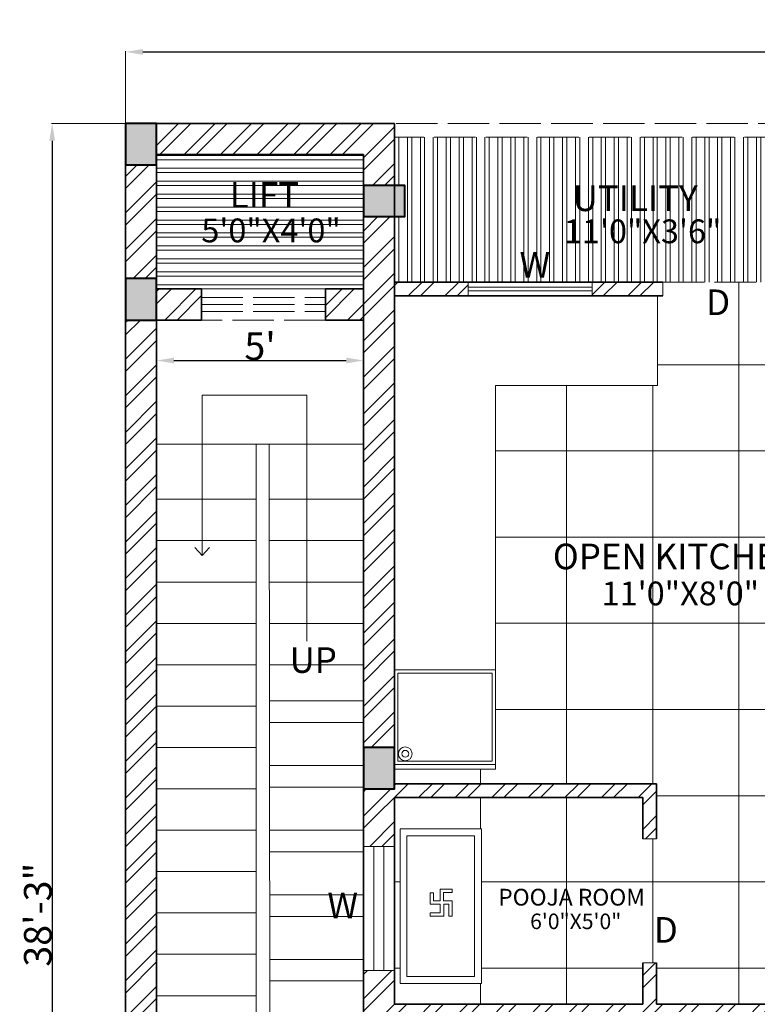
# Model space of a CAD drawing. Units: inches. Extents: x 351 to 1738, y -265 to 286.
# Tile 2 of 38: x 351 to 565, y 0 to 286. Entities that reach past the tile are written whole.
import ezdxf

# ---------------------------------------------------------------- set-up
doc = ezdxf.new("R2010")
doc.units = ezdxf.units.IN
doc.header["$MEASUREMENT"] = 0
doc.linetypes.add('ACAD_ISO02W100', pattern=[15, 12, -3])
for name, color, linetype, lineweight in [('A-ANNO-DIMS', 2, 'Continuous', 18), ('A-ANNO-SYMB', 7, 'Continuous', 18), ('A-AREA-IDEN', 7, 'Continuous', 18), ('A-COLS', 7, 'Continuous', 40), ('A-COLS-PATT', 6, 'Continuous', 13), ('A-DOOR', 3, 'Continuous', 18), ('A-DOOR-OVHD', 3, 'ACAD_ISO02W100', 13), ('A-FLOR-CASE', 9, 'Continuous', 18), ('A-FLOR-EVTR', 242, 'ACAD_ISO02W100', 18), ('A-FLOR-EVTR-PATT', 9, 'Continuous', 9), ('A-FLOR-FIXT', 9, 'Continuous', 18), ('A-FLOR-OVHD', 1, 'ACAD_ISO02W100', 18), ('A-FLOR-PATT', 9, 'Continuous', 9), ('A-FLOR-STRS', 7, 'Continuous', 18), ('A-GLAZ', 4, 'Continuous', 18), ('A-WALL', 7, 'Continuous', 35), ('A-WALL-PATT', 152, 'Continuous', 13)]:
    doc.layers.add(name, color=color, linetype=linetype, lineweight=lineweight)
doc.styles.add('Annotative', font='arial.ttf')
doc.styles.get("Standard").update_dxf_attribs({"font": 'arial.ttf'})
doc.dimstyles.get("Standard").update_dxf_attribs({"dimtxt": 8, "dimasz": 5, "dimexe": 0.18, "dimexo": 0.0625, "dimgap": 0.09, "dimtad": 1, "dimtoh": 1, "dimzin": 0, "dimdsep": 46, "dimlunit": 4, "dimtxsty": 'Standard', "dimcen": 0, "dimclre": 256, "dimadec": 0, "dimazin": 0, "dimtfac": 1, "dimtofl": 0, "dimtmove": 0, "dimatfit": 3, "dimfxl": 1, "dimtolj": 1, "dimtzin": 0, "dimlwe": -1, "dimarcsym": 0})

# ---------------------------------------------------------------- blocks, each defined once
blk = doc.blocks.new('*D2')
at = {"layer": 'A-ANNO-DIMS', "color": 0, "transparency": 16777216}
for p, q in [((382.16, 256.03), (382.16, 276.92)), ((914.16, 256.03), (914.16, 276.92))]:
    blk.add_line(p, q, dxfattribs=at)
at = {"layer": 'A-ANNO-DIMS', "color": 0, "lineweight": -2, "transparency": 16777216}
blk.add_line((387.16, 276.74), (909.16, 276.74), dxfattribs=at)
at = {"layer": 'A-ANNO-DIMS', "color": 0, "transparency": 16777216}
for points in [[(387.16, 277.57), (387.16, 275.91), (382.16, 276.74)], [(909.16, 277.57), (909.16, 275.91), (914.16, 276.74)]]:
    blk.add_solid(points, dxfattribs=at)
at = {"layer": 'Defpoints', "color": 0, "transparency": 16777216}
for p in [(914.16, 276.74), (382.16, 255.96), (914.16, 255.96)]:
    blk.add_point(p, dxfattribs=at)
at = {"layer": 'A-ANNO-DIMS', "color": 0, "transparency": 16777216, "insert": (648.16, 280.83), "char_height": 8, "attachment_point": 5}
blk.add_mtext('\\A1;44\'-4"', dxfattribs=at)
blk = doc.blocks.new('*D3')
at = {"layer": 'A-ANNO-DIMS', "color": 0, "transparency": 16777216}
for p, q in [((382.09, 255.96), (360.67, 255.96)), ((382.09, -203.04), (360.67, -203.04))]:
    blk.add_line(p, q, dxfattribs=at)
at = {"layer": 'A-ANNO-DIMS', "color": 0, "lineweight": -2, "transparency": 16777216}
blk.add_line((360.85, 250.96), (360.85, -198.04), dxfattribs=at)
at = {"layer": 'A-ANNO-DIMS', "color": 0, "transparency": 16777216}
for points in [[(360.02, 250.96), (361.69, 250.96), (360.85, 255.96)], [(360.02, -198.04), (361.69, -198.04), (360.85, -203.04)]]:
    blk.add_solid(points, dxfattribs=at)
at = {"layer": 'Defpoints', "color": 0, "transparency": 16777216}
for p in [(382.16, 255.96), (360.85, -203.04), (382.16, -203.04)]:
    blk.add_point(p, dxfattribs=at)
at = {"layer": 'A-ANNO-DIMS', "color": 0, "transparency": 16777216, "insert": (356.68, 26.46), "char_height": 8, "attachment_point": 5, "rotation": 90}
blk.add_mtext('\\A1;38\'-3"', dxfattribs=at)
blk = doc.blocks.new('*D6')
at = {"layer": 'A-ANNO-DIMS', "color": 0, "transparency": 16777216}
for p, q in [((391.16, 198.9), (391.16, 187.03)), ((451.16, 198.9), (451.16, 187.03))]:
    blk.add_line(p, q, dxfattribs=at)
at = {"layer": 'A-ANNO-DIMS', "color": 0, "lineweight": -2, "transparency": 16777216}
blk.add_line((396.16, 187.21), (446.16, 187.21), dxfattribs=at)
at = {"layer": 'A-ANNO-DIMS', "color": 0, "transparency": 16777216}
for points in [[(396.16, 188.04), (396.16, 186.37), (391.16, 187.21)], [(446.16, 188.04), (446.16, 186.37), (451.16, 187.21)]]:
    blk.add_solid(points, dxfattribs=at)
at = {"layer": 'Defpoints', "color": 0, "transparency": 16777216}
for p in [(391.16, 198.96), (451.16, 198.96), (451.16, 187.21)]:
    blk.add_point(p, dxfattribs=at)
at = {"layer": 'A-ANNO-DIMS', "color": 0, "transparency": 16777216, "insert": (421.16, 191.36), "char_height": 8, "attachment_point": 5}
blk.add_mtext("\\A1;5'", dxfattribs=at)
blk = doc.blocks.new('COL-9x12')
blk.add_lwpolyline([(0, 12), (0, 0), (9, 0), (9, 12)], close=True)
blk = doc.blocks.new('WIN-36-STAIR')
for p, q in [((3.02, 0), (3.02, 36)), ((5.92, 0), (5.92, 36))]:
    blk.add_line(p, q)
blk.add_lwpolyline([(0, 0), (0, 36), (9, 36), (9, 0)], close=True)
blk = doc.blocks.new('LIFT-DOOR-36')
for p, q in [((0, 9), (36, 9)), ((0, 6.5), (36, 6.5)), ((0, 4.5), (36, 4.5)), ((0, 2.5), (36, 2.5)), ((36, 0), (0, 0))]:
    blk.add_line(p, q)

msp = doc.modelspace()

# ---------------------------------------------------------------- hatches: boundary and pattern name
at = {"layer": 'A-COLS-PATT'}
h = msp.add_hatch(color=256, dxfattribs=at)
h.dxf.hatch_style = 1
h.paths.add_polyline_path([(460.155, 237.963), (451.155, 237.963), (451.155, 228.963), (460.155, 228.963)])
h.paths.add_polyline_path([(463.155, 237.963), (460.155, 237.963), (460.155, 228.963), (463.155, 228.963)])
h.paths.add_polyline_path([(391.155, 255.963), (382.155, 255.963), (382.155, 243.963), (391.155, 243.963)])
h.paths.add_polyline_path([(391.155, 210.963), (382.155, 210.963), (382.155, 198.963), (391.155, 198.963)])
h.paths.add_polyline_path([(391.155, -45.037), (382.155, -45.037), (382.155, -57.037), (391.155, -57.037)])
h.paths.add_polyline_path([(460.155, -45.037), (451.155, -45.037), (451.155, -57.037), (460.155, -57.037)])
h.paths.add_polyline_path([(460.155, -161.037), (451.155, -161.037), (451.155, -164.037), (451.155, -173.037), (460.155, -173.037)])
h.paths.add_polyline_path([(391.155, -161.037), (382.155, -161.037), (382.155, -173.037), (391.155, -173.037)])
h.paths.add_polyline_path([(596, -164.037), (584, -164.037), (584, -173.037), (596, -173.037)])
h.paths.add_polyline_path([(596, -50), (584, -50), (584, -59), (596, -59)])
h.paths.add_polyline_path([(596.155, 73.463), (592.155, 73.463), (592.155, 64.463), (596.155, 64.463)])
h.paths.add_polyline_path([(592.155, 73.463), (584.155, 73.463), (584.155, 64.463), (592.155, 64.463)])
h.paths.add_polyline_path([(596.155, 237.963), (584.155, 237.963), (584.155, 228.963), (596.155, 228.963)])
h.paths.add_polyline_path([(739.655, 237.963), (727.655, 237.963), (727.655, 228.963), (739.655, 228.963)])
h.paths.add_polyline_path([(883.515, 237.963), (871.515, 237.963), (871.515, 228.963), (883.515, 228.963)])
h.paths.add_polyline_path([(883.515, 73.463), (871.515, 73.463), (871.515, 64.463), (883.515, 64.463)])
h.paths.add_polyline_path([(731.655, 73.463), (727.655, 73.463), (727.655, 64.463), (731.655, 64.463)])
h.paths.add_polyline_path([(739.515, 73.463), (731.655, 73.463), (731.655, 64.463), (739.515, 64.463)])
h.paths.add_polyline_path([(883.515, -53.037), (871.515, -53.037), (871.515, -57.037), (883.515, -57.037)])
h.paths.add_polyline_path([(883.515, -48.037), (871.515, -48.037), (871.515, -53.037), (883.515, -53.037)])
h.paths.add_polyline_path([(739.515, -48.037), (727.515, -48.037), (727.515, -56.5), (727.516, -57.037), (739.515, -57.037)])
h.paths.add_polyline_path([(883.515, -164.037), (871.515, -164.037), (871.515, -173.037), (883.515, -173.037)])
h = msp.add_hatch(color=256, dxfattribs=at)
h.dxf.hatch_style = 1
h.paths.add_polyline_path([(460.155, 74.963), (451.155, 74.963), (451.155, 62.963), (460.155, 62.963)])
at = {"layer": 'A-FLOR-EVTR-PATT', "transparency": 33554559}
h = msp.add_hatch(dxfattribs=at)
h.set_pattern_fill('ANSI32', color=256, scale=10, angle=135)
h.set_pattern_definition([(180, (391.1553, 207.9627), (-2e-16, -3.75), []), (180, (389.9053, 209.2127), (-2e-16, -3.75), [])])
h.paths.add_polyline_path([(451.155, 246.963), (391.155, 246.963), (391.155, 243.963), (391.155, 207.963), (404.155, 207.963), (440.155, 207.963), (451.155, 207.963)])
at = {"layer": 'A-FLOR-PATT', "transparency": 33554559}
h = msp.add_hatch(dxfattribs=at)
h.set_pattern_fill('ANSI32', color=256, scale=10, angle=45)
h.set_pattern_definition([(90, (460.1553, 209.9627), (-3.75, 0), []), (90, (461.4053, 211.2127), (-3.75, 0), [])])
h.paths.add_polyline_path([(584.155, 237.963), (588.655, 237.963), (588.655, 251.963), (460.155, 251.963), (460.155, 237.963), (463.155, 237.963), (463.155, 228.963), (460.155, 228.963), (460.155, 209.963), (538, 209.963), (574, 209.963), (592.155, 209.963), (592.155, 228.963), (584.155, 228.963)])
h = msp.add_hatch(dxfattribs=at)
h.set_pattern_fill('ANSI37', color=256, scale=200, angle=45)
h.set_pattern_definition([(90, (460.077, -164.037), (-25, 0), []), (180, (460.077, -164.037), (-4e-15, -25), [])])
h.paths.add_polyline_path([(727.516, -57.037), (727.515, -57.037), (727.515, -56.5), (727.5, -45), (727.5, -3.5), (727.501, -2.537), (725.797, -2.537), (725.797, -3.037), (721.988, -3.037), (721.988, -2.537), (717.916, -2.537), (717.916, -3.037), (714.106, -3.037), (714.106, -2.537), (710.487, -2.537), (710.487, -3.037), (706.677, -3.037), (706.677, -2.537), (702.965, -2.537), (702.965, -3.037), (699.155, -3.037), (699.155, -2.537), (694.965, -2.537), (694.965, -3.037), (691.155, -3.037), (691.155, -2.537), (679.655, -2.537), (678.797, -2.537), (677.776, -2.537), (676.723, -2.537), (652.655, -2.537), (651.799, -2.537), (650.778, -2.537), (649.725, -2.537), (625.877, -2.537), (624.879, -2.537), (623.857, -2.537), (622.804, -2.537), (596.155, -2.537), (596.155, -3.537), (460.155, -3.537), (460.155, -81.037), (460.077, -99.07), (460.077, -133.967), (460.155, -152.037), (460.155, -164.037), (485.277, -164.037), (545.277, -164.037), (727.655, -164.037)])
h.paths.add_polyline_path([(584, -59), (584, -50), (596, -50), (596, -59)], flags=16)
h.paths.add_polyline_path([(905.155, 204.963), (731.655, 204.963), (731.655, 73.463), (739.515, 73.463), (739.515, 64.463), (731.655, 64.463), (731.655, -3.5), (727.655, -3.5), (727.655, -3.537), (727.5, -45), (731.655, -45), (731.655, -48.037), (739.515, -48.037), (739.515, -53.037), (754, -53.037), (754, -57.037), (748.655, -57.037), (748.655, -147.037), (815.655, -147.037), (815.655, -138.5), (819.655, -138.5), (819.655, -102.5), (815.655, -102.5), (815.655, -57.037), (790, -57.037), (790, -53.037), (871.515, -53.037), (871.515, -48.037), (883.515, -48.037), (883.515, -53.037), (905.155, -53.037)])
h.paths.add_polyline_path([(871.515, 64.463), (871.515, 73.463), (883.515, 73.463), (883.515, 64.463)], flags=16)
h.paths.add_polyline_path([(727.655, 64.463), (685.515, 64.463), (685.515, 186.963), (638.155, 186.963), (638.155, 88.463), (596.155, 88.463), (596.155, 64.463), (584.155, 64.463), (584.155, 73.463), (592.155, 73.463), (592.155, 205.963), (574, 205.963), (574, 209.963), (538, 209.963), (538, 205.963), (536.5, 205.963), (536.5, 180), (489.5, 180), (489.5, 68.655), (460.155, 68.655), (460.155, 64.463), (536.155, 64.463), (536.155, 48.463), (532.155, 48.463), (532.155, 60.463), (460.155, 60.463), (460.155, 0.463), (532.155, 0.463), (532.155, 12.463), (536.155, 12.463), (536.155, 0.463), (596.155, 0.463), (596.155, -0.537), (622.655, -0.537), (623.655, -0.537), (624.655, -0.537), (625.655, -0.537), (649.655, -0.537), (650.576, -0.537), (651.576, -0.537), (652.576, -0.537), (676.655, -0.537), (677.574, -0.537), (678.574, -0.537), (679.574, -0.537), (691.155, -0.537), (691.155, -0.037), (694.965, -0.037), (694.965, -0.537), (699.155, -0.537), (699.155, -0.037), (702.965, -0.037), (702.965, -0.537), (706.677, -0.537), (706.677, -0.037), (710.487, -0.037), (710.487, -0.537), (714.106, -0.537), (714.106, -0.037), (717.916, -0.037), (717.916, -0.537), (721.988, -0.537), (721.988, -0.037), (725.797, -0.037), (725.797, -0.537), (727.655, -0.537)])
h.paths.add_polyline_path([(485.401, 6.538), (461.783, 6.538), (461.783, 51.327), (485.401, 51.327)], flags=16)
h.paths.add_polyline_path([(483.401, 8.538), (463.783, 8.538), (463.783, 49.327), (483.401, 49.327)], flags=0)
h.paths.add_polyline_path([(476.907, 30.5), (476.907, 29.5), (476.907, 26), (475.907, 26), (475.907, 29.5), (474.449, 29.5), (474.449, 26), (473.449, 26), (470.5, 26), (470.5, 27), (473.449, 27), (473.449, 29.5), (470.5, 29.5), (470.5, 32.758), (471.5, 32.758), (471.5, 30.5), (473.407, 30.5), (473.407, 32.897), (473.407, 33.897), (476.907, 33.897), (476.907, 32.897), (474.407, 32.897), (474.407, 30.5)], flags=0)
h = msp.add_hatch(dxfattribs=at)
h.set_pattern_fill('ANSI32', color=256, scale=50, angle=135)
h.set_pattern_definition([(180, (386.155, -199.037), (-2e-15, -18.75), []), (180, (379.905, -192.787), (-2e-15, -18.75), [])])
h.paths.add_polyline_path([(451.234, -133.967), (460.077, -133.967), (460.077, -99.07), (451.234, -99.07), (451.155, -81.037), (451.155, 98.963), (423.885, 98.963), (424, -81.037), (419, -81.037), (391.155, -81.037), (386.155, -81.037), (386.155, -161.037), (391.155, -161.037), (391.155, -173.037), (386.155, -173.037), (386.155, -199.037), (910.155, -199.037), (910.155, -173.037), (545.277, -173.037), (545.277, -164.037), (485.277, -164.037), (485.277, -173.037), (451.155, -173.037), (451.155, -161.037), (451.155, -152.037)])
at = {"layer": 'A-WALL-PATT'}
h = msp.add_hatch(dxfattribs=at)
h.set_pattern_fill('ANSI32', color=256, scale=20)
h.set_pattern_definition([(45, (382.155, -173.037), (-5.3033, 5.3033), []), (45, (385.691, -173.037), (-5.3033, 5.3033), [])])
h.paths.add_polyline_path([(391.155, -57.037), (382.155, -57.037), (382.155, -81.037), (391.155, -81.037)])
h.paths.add_polyline_path([(391.155, 198.963), (382.155, 198.963), (382.155, -45.037), (391.155, -45.037)])
h.paths.add_polyline_path([(391.155, 243.963), (382.155, 243.963), (382.155, 237.963), (382.155, 210.963), (391.155, 210.963)])
h.paths.add_polyline_path([(460.155, 255.963), (391.155, 255.963), (391.155, 246.963), (451.155, 246.963), (451.155, 237.963), (460.155, 237.963), (460.155, 251.963)])
h.paths.add_polyline_path([(404.155, 207.963), (391.155, 207.963), (391.155, 198.963), (404.155, 198.963)])
h.paths.add_polyline_path([(451.155, 207.963), (440.155, 207.963), (440.155, 198.963), (451.155, 198.963)])
h.paths.add_polyline_path([(460.155, 228.963), (451.155, 228.963), (451.155, 74.963), (460.155, 74.963), (460.155, 97.5)])
h.paths.add_polyline_path([(460.155, 60.463), (532.155, 60.463), (532.155, 48.463), (536.155, 48.463), (536.155, 64.463), (460.155, 64.463), (460.155, 62.963), (451.155, 62.963), (451.155, 46.258), (460.155, 46.258)])
h.paths.add_polyline_path([(460.155, -3.537), (596.155, -3.537), (596.155, 0.463), (536.155, 0.463), (536.155, 12.463), (532.155, 12.463), (532.155, 0.463), (460.155, 0.463), (460.155, 10.258), (451.155, 10.258), (451.155, -45.037), (460.155, -45.037)])
h.paths.add_polyline_path([(460.155, -57.037), (451.155, -57.037), (451.155, -81.037), (460.155, -81.037)])
h.paths.add_polyline_path([(460.155, -152.037), (451.155, -152.037), (451.155, -161.037), (460.155, -161.037)])
h.paths.add_polyline_path([(485.277, -164.037), (460.155, -164.037), (460.155, -164.5), (460.155, -173.037), (485.277, -173.037)])
h.paths.add_polyline_path([(584, -164.037), (545.277, -164.037), (545.277, -173.037), (584, -173.037)])
h.paths.add_polyline_path([(631.58, -164.037), (596, -164.037), (596, -173.037), (631.58, -173.037)])
h.paths.add_polyline_path([(871.515, -164.037), (819.655, -164.037), (819.655, -138.5), (815.655, -138.5), (815.655, -164.037), (691.58, -164.037), (691.58, -173.037), (871.515, -173.037)])
h.paths.add_polyline_path([(731.655, -57.037), (727.516, -57.037), (727.655, -164.037), (731.655, -164.037)])
h.paths.add_polyline_path([(914.155, -138), (905.155, -138), (905.155, -164.037), (883.515, -164.037), (883.515, -173.037), (914.155, -173.037)])
h.paths.add_polyline_path([(914.155, -30.189), (905.155, -30.189), (905.155, -53.037), (883.515, -53.037), (883.515, -57.037), (905.155, -57.037), (905.155, -102), (914.155, -102)])
h.paths.add_polyline_path([(871.515, -53.037), (790, -53.037), (790, -57.037), (815.655, -57.037), (815.655, -102.5), (819.655, -102.5), (819.655, -57.037), (871.515, -57.037)])
h.paths.add_polyline_path([(914.155, 120.993), (905.155, 120.993), (905.155, 29.811), (914.155, 29.811)])
h.paths.add_polyline_path([(731.655, 64.463), (727.655, 64.463), (727.655, -3.5), (731.655, -3.5)])
h.paths.add_polyline_path([(481.5, 209.963), (460.155, 209.963), (460.155, 205.963), (481.5, 205.963)])
h.paths.add_polyline_path([(538, 209.963), (517.5, 209.963), (517.5, 205.963), (538, 205.963)])
h.paths.add_polyline_path([(592.155, 209.963), (574, 209.963), (574, 205.963), (592.155, 205.963)])
h.paths.add_polyline_path([(596.155, 228.963), (592.155, 228.963), (592.155, 73.463), (596.155, 73.463)])
h.paths.add_polyline_path([(614, 237.963), (596.155, 237.963), (596.155, 228.963), (614, 228.963)])
h.paths.add_polyline_path([(677, 237.963), (650, 237.963), (650, 228.963), (677, 228.963)])
h.paths.add_polyline_path([(727.655, 237.963), (713, 237.963), (713, 228.963), (727.655, 228.963)])
h.paths.add_polyline_path([(871.515, 237.963), (739.655, 237.963), (739.655, 228.963), (871.515, 228.963)])
h.paths.add_polyline_path([(731.655, 228.963), (727.655, 228.963), (727.655, 73.463), (731.655, 73.463)])
h.paths.add_polyline_path([(914.155, 237.963), (883.515, 237.963), (883.515, 228.963), (905.155, 228.963), (905.155, 180.993), (914.155, 180.993)])

# ---------------------------------------------------------------- linework, layer by layer
at = {"layer": 'A-ANNO-SYMB'}
for points in [[(434.684, 105.774), (434.684, 177.128), (404.353, 177.128), (404.353, 130.616)], [(402.248, 133.018), (404.353, 130.616), (406.457, 133.018)]]:
    msp.add_lwpolyline(points, dxfattribs=at)
at = {"layer": 'A-DOOR'}
for p, q in [((538, 209.963), (538, 205.963)), ((536.155, 48.463), (532.155, 48.463)), ((536.155, 12.463), (532.155, 12.463))]:
    msp.add_line(p, q, dxfattribs=at)
at = {"layer": 'A-DOOR-OVHD'}
msp.add_line((538, 209.963), (574, 209.963), dxfattribs=at)
at = {"layer": 'A-FLOR-CASE'}
for p, q in [((536.5, 180), (536.5, 205.963)), ((489.5, 68.655), (489.5, 180)), ((489.5, 180), (536.5, 180)), ((460.155, 68.655), (489.5, 68.655))]:
    msp.add_line(p, q, dxfattribs=at)
for points in [[(461.783, 6.538), (485.401, 6.538), (485.401, 51.327), (461.783, 51.327)], [(463.783, 8.538), (483.401, 8.538), (483.401, 49.327), (463.783, 49.327)], [(475.907, 26), (476.907, 26), (476.907, 30.5), (474.407, 30.5), (474.407, 32.897), (476.907, 32.897), (476.907, 33.897), (473.407, 33.897), (473.407, 30.5), (471.5, 30.5), (471.5, 32.758), (470.5, 32.758), (470.5, 29.5), (473.449, 29.5), (473.449, 27), (470.5, 27), (470.5, 26), (474.449, 26), (474.449, 29.5), (475.907, 29.5)]]:
    msp.add_lwpolyline(points, close=True, dxfattribs=at)
at = {"layer": 'A-FLOR-FIXT'}
for points in [[(460.155, 70), (489.5, 70), (489.5, 97.5), (460.155, 97.5)], [(461.155, 71), (488.5, 71), (488.5, 96.5), (461.155, 96.5)]]:
    msp.add_lwpolyline(points, close=True, dxfattribs=at)
for radius in [2, 1]:
    msp.add_circle((463.272, 73.125), radius, dxfattribs=at)
at = {"layer": 'A-FLOR-OVHD'}
for p, q in [((592.655, 255.963), (460.155, 255.963)), ((588.655, 251.963), (460.155, 251.963)), ((588.655, 251.963), (460.155, 251.963))]:
    msp.add_line(p, q, dxfattribs=at)
at = {"layer": 'A-FLOR-STRS'}
for p, q in [((391.155, 162.963), (451.155, 162.963)), ((420, -81.037), (420, 162.963)), ((423.845, 162.963), (424, -81.037)), ((391.155, 146.963), (420, 146.963)), ((423.855, 146.963), (451.155, 146.963)), ((391.155, 134.963), (420, 134.963)), ((423.863, 134.963), (451.155, 134.963)), ((391.155, 122.963), (420, 122.963)), ((423.87, 122.963), (451.155, 122.963)), ((391.155, 110.963), (420, 110.963)), ((423.878, 110.963), (451.155, 110.963)), ((391.155, 98.963), (420, 98.963)), ((423.885, 98.963), (451.155, 98.963)), ((391.155, 86.963), (420, 86.963)), ((391.155, 74.963), (420, 74.963)), ((391.155, 62.963), (420, 62.963)), ((391.155, 50.963), (420, 50.963)), ((391.155, 38.963), (420, 38.963)), ((391.155, 26.963), (420, 26.963)), ((391.155, 14.963), (420, 14.963)), ((391.155, 2.963), (420, 2.963))]:
    msp.add_line(p, q, dxfattribs=at)
at = {"layer": 'A-GLAZ'}
for p, q in [((481.5, 208.463), (517.5, 208.463)), ((481.5, 207.463), (517.5, 207.463))]:
    msp.add_line(p, q, dxfattribs=at)
msp.add_lwpolyline([(517.5, 205.963), (517.5, 209.963), (481.5, 209.963), (481.5, 205.963)], close=True, dxfattribs=at)
at = {"layer": 'A-WALL'}
for p, q in [((382.155, 255.963), (382.155, 237.963)), ((460.155, 255.963), (382.155, 255.963)), ((382.155, 255.963), (382.155, -81.037)), ((391.155, 255.963), (391.155, 207.963)), ((460.155, 255.963), (460.155, 64.463)), ((460.155, 251.963), (460.155, 237.963)), ((451.155, 246.963), (391.155, 246.963)), ((451.155, 246.963), (451.155, -81.037)), ((460.155, 228.963), (460.155, 209.963)), ((460.155, 209.963), (538, 209.963)), ((404.155, 207.963), (391.155, 207.963)), ((404.155, 198.963), (404.155, 207.963)), ((451.155, 207.963), (440.155, 207.963)), ((440.155, 207.963), (440.155, 198.963)), ((460.155, 205.963), (538, 205.963)), ((404.155, 198.963), (391.155, 198.963)), ((391.155, 198.963), (391.155, -81.037)), ((451.155, 198.963), (440.155, 198.963)), ((460.155, 64.463), (536.155, 64.463)), ((536.155, 64.463), (536.155, 48.463)), ((460.155, 60.463), (532.155, 60.463)), ((460.155, 60.463), (460.155, 0.463)), ((532.155, 60.463), (532.155, 48.463)), ((532.155, 12.463), (532.155, 0.463)), ((536.155, 12.463), (536.155, 0.463)), ((460.155, 0.463), (532.155, 0.463)), ((536.155, 0.463), (596.155, 0.463))]:
    msp.add_line(p, q, dxfattribs=at)

# ---------------------------------------------------------------- block references
at = {"layer": 'A-COLS'}
for p in [(382.155, 243.963), (382.155, 198.963), (451.155, 62.963)]:
    msp.add_blockref('COL-9x12', p, dxfattribs=at)
at = {"layer": 'A-COLS', "rotation": 90.00000000000033}
msp.add_blockref('COL-9x12', (463.155, 228.962), dxfattribs=at)
at = {"layer": 'A-FLOR-EVTR'}
msp.add_blockref('LIFT-DOOR-36', (404.155, 198.963), dxfattribs=at)
at = {"layer": 'A-GLAZ'}
msp.add_blockref('WIN-36-STAIR', (451.155, 10.258), dxfattribs=at)

# ---------------------------------------------------------------- texts
at = {"layer": 'A-ANNO-SYMB', "style": 'Annotative'}
for s, height, p in [('W', 7.433, (496.428, 211.266)), ('D', 7.433, (550.549, 200.387)), ('UP', 7.4326, (429.71, 96.607)), ('W', 7.433, (440.683, 25.438)), ('D', 7.433, (535.375, 18.333))]:
    msp.add_text(s, height=height, dxfattribs=at).set_placement(p)
at = {"layer": 'A-AREA-IDEN', "style": 'Annotative'}
for s, height, p in [('LIFT', 7.4326, (412.358, 231.521)), ('UTILITY', 7.4326, (511.816, 230.558)), ('5\'0"X4\'0"', 6.9014, (404.124, 221.498)), ('11\'0"X3\'6"', 6.9014, (509.302, 221.235)), ('OPEN KITCHEN', 7.43256, (506.097, 126.656)), ('11\'0"X8\'0"', 6.9014, (520.25, 116.199)), ('POOJA ROOM', 4.8596, (490.247, 29.11)), ('6\'0"X5\'0"', 4.5123, (499.5, 22.273))]:
    msp.add_text(s, height=height, dxfattribs=at).set_placement(p)

# ---------------------------------------------------------------- dimensions: what is measured, and where the dimension line sits
at = {"layer": 'A-ANNO-DIMS'}
dim = msp.add_linear_dim(base=(914.155, 276.74), p1=(382.155, 255.963), p2=(914.155, 255.963), dimstyle='Standard', override={"dimclrd": 0, "dimclre": 0, "dimclrt": 0}, dxfattribs=at)
dim.commit()
dim.dimension.update_dxf_attribs({"geometry": '*D2', "text_midpoint": (648.155, 280.83)})
dim = msp.add_linear_dim(base=(360.852, -203.037), p1=(382.155, 255.963), p2=(382.155, -203.037), angle=90, dimstyle='Standard', override={"dimclrd": 0, "dimclre": 0, "dimclrt": 0}, dxfattribs=at)
dim.commit()
dim.dimension.update_dxf_attribs({"geometry": '*D3', "text_midpoint": (360.852, 26.463), "dimtype": 160})
dim = msp.add_linear_dim(base=(451.155, 187.205), p1=(391.155, 198.963), p2=(451.155, 198.963), dimstyle='Standard', override={"dimclrd": 0, "dimclre": 0, "dimclrt": 0}, dxfattribs=at)
dim.commit()
dim.dimension.update_dxf_attribs({"geometry": '*D6', "text_midpoint": (421.155, 187.205), "dimtype": 160})

doc.saveas('drawing.dxf')
